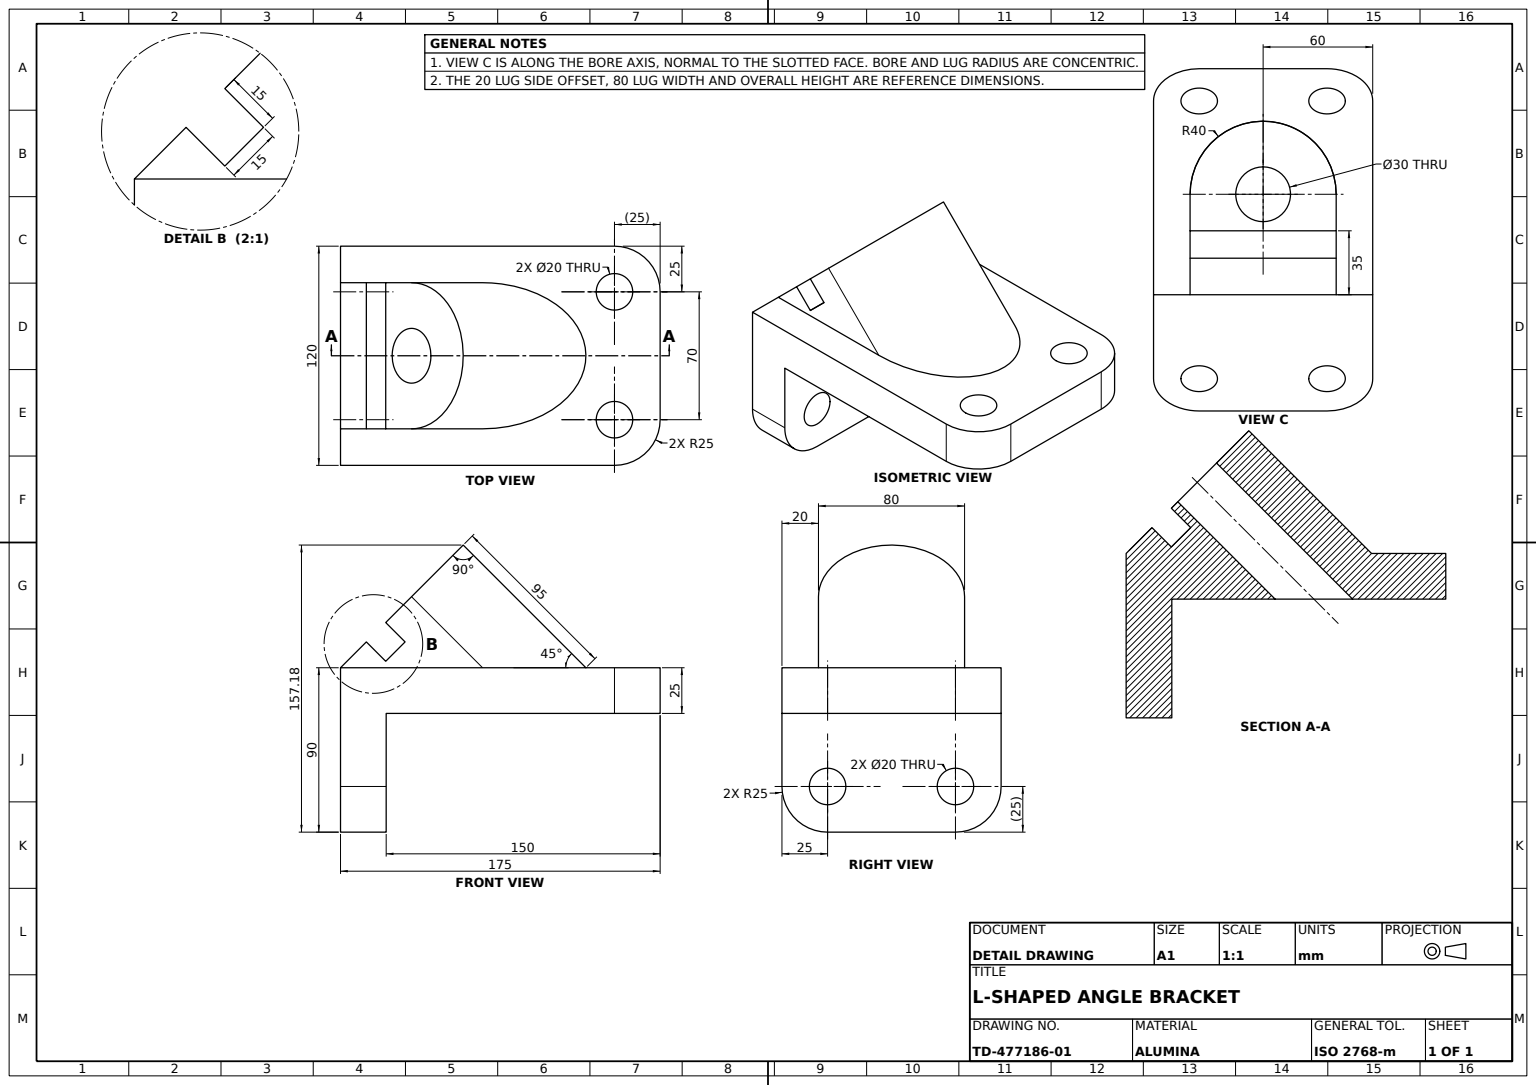
SolidWorks part; units mm, degrees
material "Alumina"
ref_plane "Front Plane" through (0, 0, 0) normal (0, 0, 1) x (1, 0, 0)
ref_plane "Top Plane" through (0, 0, 0) normal (0, 1, 0) x (1, 0, 0)
ref_plane "Right Plane" through (0, 0, 0) normal (1, 0, 0) x (0, 0, -1)
sketch "Base Plate Sketch" plane through (0, 0, 0) normal (0, 0, 1) x (1, 0, 0)
  line L1 (-35, -90) -> (35, -90)
  line L2 (-60, -65) -> (-60, 0)
  line L3 (-60, 0) -> (60, 0)
  line L4 (60, -65) -> (60, 0)
  arc A0 (35, -90) -> (60, -65) centre (35, -65) ccw
  arc A1 (-35, -90) -> (-60, -65) centre (-35, -65) cw
  point P4 (0, 0)
  dimension "D3" = 25
  dimension "D1" = 90
  dimension "D2" = 120
extrude "Base Plate" add sketch "Base Plate Sketch" against normal blind 25
sketch "Upright Flange Sketch" plane through (0, 0, 0) normal (1, 0, 0) x (0, 0, -1)
  line L0 (25, 0) -> (175, 0)
  line L1 (175, 0) -> (175, -25)
  line L2 (175, -25) -> (25, -25)
  line L3 (25, -65) -> (25, 0) construction
  line L4 (25, -25) -> (25, 0)
  dimension "D1" = 25
  dimension "D2" = 150
extrude "Upright Flange" add sketch "Upright Flange Sketch" along normal mid plane 120
sketch "Base Holes Sketch" plane through (0, 0, 0) normal (0, 0, 1) x (1, 0, 0)
  circle A1 centre (35, -65) radius 10
  arc A3 (35, -90) -> (60, -65) centre (35, -65) ccw construction
  circle A4 centre (-35, -65) radius 10
  arc A5 (-60, -65) -> (-35, -90) centre (-35, -65) ccw construction
  dimension "D2" = 20
extrude "Base Mounting Holes" cut sketch "Base Holes Sketch" against normal up to next
sketch "Lug Support Sketch" plane through (0, 0, 0) normal (1, 0, 0) x (0, 0, -1)
  line L0 (0, 0) -> (67.1751, 67.1751)
  line L1 (67.1751, 67.1751) -> (134.3503, 0)
  line L2 (175, 0) -> (0, 0) construction
  line L3 (134.3503, 0) -> (0, 0)
  dimension "D1" = 45
  dimension "D2" = 95
extrude "Lug Support" add sketch "Lug Support Sketch" along normal mid plane 120
sketch "Lug Clearance Sketch" plane through (0, 0, 0) normal (0, 0.7071, 0.7071) x (1, 0, 0)
  line L0 (-40, 0) -> (-40, 55)
  line L1 (60, 0) -> (-60, 0) construction
  line L2 (40, 55) -> (40, 0)
  line L3 (40, 0) -> (-40, 0)
  line L4 (60, 95) -> (-60, 95) construction
  arc A0 (-40, 55) -> (40, 55) centre (0, 55) cw
  line M5 (-60, 95) -> (-60, 0)
  line M6 (-60, 0) -> (60, 0)
  line M7 (60, 0) -> (60, 95)
  line M8 (60, 95) -> (-60, 95)
  dimension "D1" = 80
extrude "Lug Clearance Cut" cut sketch "Lug Clearance Sketch" against normal up to surface contours A0 L2 M8 M6 M7 | L0 A0 M8 M5 M6
sketch "Lug Bore Sketch" plane through (0, 0, 0) normal (0, 0.7071, 0.7071) x (1, 0, 0)
  circle A0 centre (0, 55) radius 15
  arc A1 (40, 55) -> (-40, 55) centre (0, 55) ccw construction
  dimension "D1" = 30
extrude "Lug Bore Ø30" cut sketch "Lug Bore Sketch" against normal up to next
sketch "Lug Slot Sketch" plane through (0, 0, 0) normal (0, 0.7071, 0.7071) x (1, 0, 0)
  line L7 (-40, 55) -> (-40, 0) construction
  line L8 (-40, 20) -> (40, 20)
  line L9 (-40, 20) -> (-40, 35)
  line L10 (-40, 35) -> (40, 35)
  line L11 (40, 20) -> (40, 35)
  line L12 (40, 55) -> (40, 0) construction
  line L13 (60, 0) -> (40, 0) construction
  dimension "D1" = 15
  dimension "D2" = 20
extrude "Lug Slot" cut sketch "Lug Slot Sketch" against normal blind 15 contours L8 L11 L10 L9
fillet "Flange Corner Fillets R25" radius 25 2 edges at (-60, -12.5, -175) (60, -12.5, -175)
sketch "Flange Holes Sketch" plane through (0, 0, 0) normal (0, 1, 0) x (1, 0, 0)
  circle A0 centre (-35, 150) radius 10
  circle A1 centre (35, 150) radius 10
  arc A2 (-35, 175) -> (-60, 150) centre (-35, 150) ccw construction
  arc A3 (60, 150) -> (35, 175) centre (35, 150) ccw construction
  dimension "D1" = 20
extrude "Flange Mounting Holes" cut sketch "Flange Holes Sketch" against normal up to next
